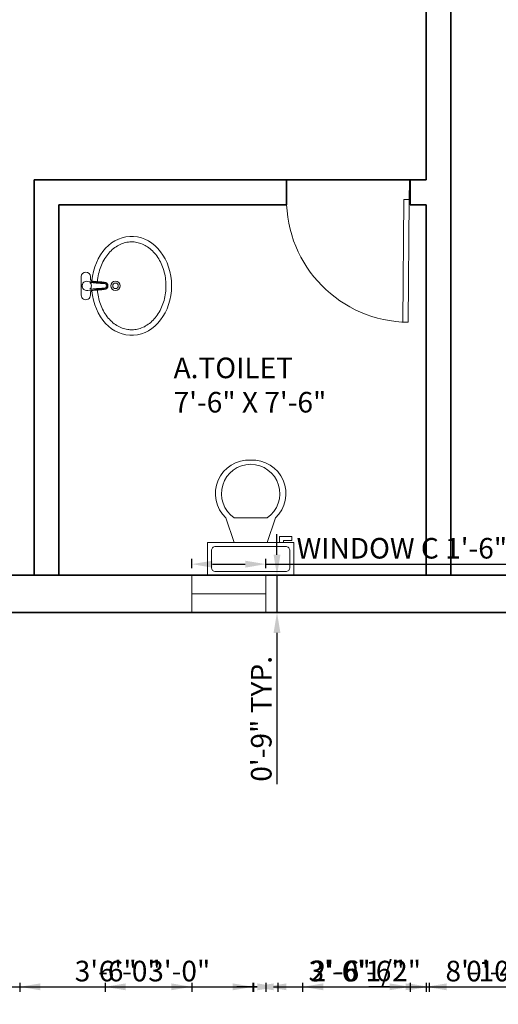
# Model space of a CAD drawing. Units: inches. Extents: x -100 to 766, y -562 to 63.
# Tile 2 of 11: x 152 to 268, y -562 to -323. Entities that reach past the tile are written whole.
import ezdxf

# ---------------------------------------------------------------- set-up
doc = ezdxf.new("R2010")
doc.units = ezdxf.units.IN
for name, color, linetype, lineweight in [('A-ANNO-DIMS', 2, 'Continuous', 18), ('A-AREA-IDEN', 7, 'Continuous', 18), ('A-DOOR', 3, 'Continuous', 18), ('A-FLOR-FIXT', 8, 'Continuous', 18), ('A-GLAZ', 4, 'Continuous', 18), ('A-WALL', 7, 'Continuous', 35)]:
    doc.layers.add(name, color=color, linetype=linetype, lineweight=lineweight)
doc.styles.get("Standard").update_dxf_attribs({"font": 'arial.ttf'})
doc.dimstyles.new('ISO-25', dxfattribs={"dimtxt": 5, "dimasz": 5, "dimexe": 1.25, "dimexo": 0.625, "dimtad": 1, "dimlunit": 3, "dimtxsty": 'Standard', "dimcen": 2.5, "dimadec": 0, "dimazin": 0, "dimtfac": 1, "dimtmove": 0, "dimatfit": 3, "dimfxl": 1, "dimfxlon": 1, "dimarcsym": 0})

# ---------------------------------------------------------------- blocks, each defined once
blk = doc.blocks.new('*U2')
for p, q in [((0, 0), (0, -6)), ((40, 0), (40, -6))]:
    blk.add_line(p, q)
blk.add_lwpolyline([(0, 0), (0, 40), (1.75, 40), (1.75, 0)], close=True)
blk.add_arc((0, 0), 40, 0, 90)
blk = doc.blocks.new('*U4')
for p, q in [((9.5, -6), (9.5, -2)), ((-10, -8.5), (-8, -8.5)), ((-10, -9.5), (-10, -8.5)), ((-7, -9.5), (-10, -9.5)), ((-8, -8.5), (-8, -8)), ((-7, -8), (-7, -9.5)), ((-4, -8), (-6, -14)), ((4, -8), (6, -14)), ((4, -14), (-4, -14))]:
    blk.add_line(p, q)
blk.add_lwpolyline([(10.5, -8), (10.5, 0), (-10.5, 0), (-10.5, -8)], close=True)
for points in [[(-9.5, -2), (-9.5, -6)], [(8.5, -1), (-8.5, -1)], [(-8.5, -7), (8.5, -7)]]:
    blk.add_lwpolyline(points)
for centre, radius, start, end in [((-8.625, -1.875), 0.8839, 81.8699, 188.1301), ((8.625, -1.875), 0.8839, 351.8699, 98.1301), ((-8.625, -6.125), 0.8839, 171.869898, 278.1301), ((8.625, -6.125), 0.8839, 261.8699, 8.1301), ((-0.4772, -19.9188), 8.0953, 133.01722, 273.38), ((0.0374, -19.8731), 7.127, 124.50543, 269.7), ((-0.0373, -19.8731), 7.127, 270.3, 55.4946), ((0.4773, -19.9188), 8.0953, 266.62, 46.9828)]:
    blk.add_arc(centre, radius, start, end)
blk = doc.blocks.new('A$C359865C9')
for p, q in [((0.26, 0.5858), (0.38, 0.5858)), ((0.26, 0.5258), (0.272, 0.5258)), ((0.368, 0.5258), (0.3809, 0.5258))]:
    blk.add_line(p, q)
for radius in [0.03, 0.018]:
    blk.add_circle((0.3201, 0.3632), radius)
for centre, radius, start, end in [((0.26, 0.5558), 0.03, 90.00613, 270.00613), ((0.32, 0.5495), 0.03, 348.15369, 191.84631), ((0.38, 0.5558), 0.03, 270.00613, 89.98161), ((0.272, 0.5078), 0.018, 0.00613, 90.00613), ((0.32, 0.5495), 0.03, 222.45226, 317.54774), ((0.368, 0.5078), 0.018, 90.00613, 180.00613), ((0.3201, 0.4358), 0.024, 180.00613, 0.00613), ((0.3201, 0.4358), 0.0204, 180.00613, 0.00613), ((0.3201, 0.4358), 0.0144, 180.00613, 0.00613)]:
    blk.add_arc(centre, radius, start, end)
at = {"extrusion": (0, 0, -1)}
blk.add_ellipse((0.3199, 0.5826), major_axis=(-0.00812, 0), ratio=0.392595, dxfattribs=at)
at = {"ltscale": 100, "extrusion": (0, 0, -1)}
blk.add_ellipse((0.3201, 0.258), major_axis=(0.3216, 0), ratio=0.80597, start_param=-1.471508, end_param=4.612925, dxfattribs=at)
for points, knots in [([(0.2907, 0.5434), (0.2946, 0.498), (0.2952, 0.4908), (0.2965, 0.4761), (0.2971, 0.4686), (0.2983, 0.4536), (0.2989, 0.4461), (0.2995, 0.4378), (0.2996, 0.4369), (0.2996, 0.4361)], [2.511178, 2.511178, 2.511178, 2.511178, 20.495008, 20.495008, 39.297594, 39.297594, 58.10018, 58.10018, 60.208758, 60.208758, 60.208758, 60.208758]), ([(0.2979, 0.5293), (0.298, 0.528), (0.2981, 0.5267), (0.2988, 0.5184), (0.2993, 0.5127), (0.3005, 0.4986), (0.301, 0.4933), (0.3014, 0.4884), (0.3015, 0.4875), (0.3017, 0.4857), (0.3017, 0.485), (0.3019, 0.4827), (0.3021, 0.4812), (0.3026, 0.4756), (0.3029, 0.4716), (0.3037, 0.4621), (0.3041, 0.4568), (0.3049, 0.4464), (0.3053, 0.4415), (0.3056, 0.4365)], [4.643985, 4.643985, 4.643985, 4.643985, 5.282102, 5.282102, 8.976667, 8.976667, 16.365798, 16.365798, 18.536065, 18.536065, 20.434607, 20.434607, 24.231692, 24.231692, 34.371999, 34.371999, 47.807513, 47.807513, 60.208758, 60.208758, 60.208758, 60.208758]), ([(0.3422, 0.5293), (0.3421, 0.528), (0.342, 0.5267), (0.3412, 0.5184), (0.3408, 0.5127), (0.3395, 0.4986), (0.3391, 0.4933), (0.3387, 0.4884), (0.3386, 0.4875), (0.3384, 0.4857), (0.3383, 0.485), (0.3381, 0.4827), (0.338, 0.4812), (0.3375, 0.4756), (0.3372, 0.4716), (0.3364, 0.4621), (0.336, 0.4568), (0.3352, 0.4464), (0.3348, 0.4415), (0.3345, 0.4365)], [4.643985, 4.643985, 4.643985, 4.643985, 5.282102, 5.282102, 8.976667, 8.976667, 16.365798, 16.365798, 18.536065, 18.536065, 20.434607, 20.434607, 24.231692, 24.231692, 34.371999, 34.371999, 47.807513, 47.807513, 60.208758, 60.208758, 60.208758, 60.208758]), ([(0.3494, 0.5434), (0.3455, 0.498), (0.3449, 0.4908), (0.3436, 0.4761), (0.343, 0.4686), (0.3418, 0.4536), (0.3412, 0.4461), (0.3406, 0.4378), (0.3405, 0.4369), (0.3404, 0.4361)], [2.511178, 2.511178, 2.511178, 2.511178, 20.495008, 20.495008, 39.297594, 39.297594, 58.10018, 58.10018, 60.208758, 60.208758, 60.208758, 60.208758]), ([(0.3475, 0.4801), (0.3477, 0.4801), (0.3479, 0.4801), (0.3648, 0.4788), (0.3813, 0.4763), (0.4136, 0.4692), (0.4293, 0.4645), (0.4593, 0.4531), (0.4737, 0.4464), (0.5006, 0.4312), (0.5131, 0.4227), (0.5361, 0.4042), (0.5465, 0.3942), (0.5649, 0.3732), (0.5729, 0.3622), (0.5864, 0.3393), (0.5918, 0.3275), (0.6, 0.3036), (0.6029, 0.2914), (0.6059, 0.2669), (0.6061, 0.2545), (0.6039, 0.2301), (0.6015, 0.218), (0.5941, 0.1942), (0.5892, 0.1825), (0.5768, 0.1597), (0.5693, 0.1486), (0.552, 0.1275), (0.5422, 0.1174), (0.5203, 0.0986), (0.5083, 0.0899), (0.4825, 0.0741), (0.4686, 0.0671), (0.4396, 0.0549), (0.4243, 0.0498), (0.3929, 0.0418), (0.3767, 0.0388), (0.3439, 0.0352), (0.3273, 0.0344), (0.2942, 0.0353), (0.2776, 0.0369), (0.2452, 0.0422), (0.2293, 0.046), (0.1987, 0.0556), (0.1839, 0.0615), (0.156, 0.0751), (0.1428, 0.0828), (0.1184, 0.0997), (0.1071, 0.109), (0.0869, 0.1288), (0.078, 0.1393), (0.0625, 0.1611), (0.0559, 0.1725), (0.0454, 0.1957), (0.0415, 0.2076), (0.036, 0.2317), (0.0346, 0.2438), (0.0345, 0.2566), (0.0345, 0.2573), (0.0345, 0.258), (0.0345, 0.2664), (0.0351, 0.2749), (0.0382, 0.2956), (0.0413, 0.3078), (0.0502, 0.3317), (0.0559, 0.3434), (0.0699, 0.3661), (0.0782, 0.377), (0.0972, 0.3978), (0.1079, 0.4076), (0.1313, 0.4257), (0.1441, 0.434), (0.1714, 0.4488), (0.186, 0.4553), (0.2163, 0.4662), (0.2321, 0.4706), (0.2628, 0.4769), (0.2776, 0.479), (0.2925, 0.4801)], [1.664851, 1.664851, 1.664851, 1.664851, 1.666804, 1.666804, 1.838807, 1.838807, 2.01081, 2.01081, 2.182814, 2.182814, 2.354817, 2.354817, 2.52682, 2.52682, 2.698824, 2.698824, 2.870827, 2.870827, 3.04283, 3.04283, 3.214834, 3.214834, 3.384783, 3.384783, 3.554732, 3.554732, 3.724681, 3.724681, 3.89463, 3.89463, 4.064578, 4.064578, 4.234527, 4.234527, 4.404476, 4.404476, 4.574425, 4.574425, 4.744374, 4.744374, 4.914323, 4.914323, 5.084272, 5.084272, 5.254221, 5.254221, 5.42417, 5.42417, 5.594119, 5.594119, 5.764068, 5.764068, 5.934016, 5.934016, 6.103965, 6.103965, 6.273914, 6.273914, 6.283185, 6.283185, 6.283185, 6.401959, 6.401959, 6.573962, 6.573962, 6.745965, 6.745965, 6.917969, 6.917969, 7.089972, 7.089972, 7.261975, 7.261975, 7.433979, 7.433979, 7.605982, 7.605982, 7.759676, 7.759676, 7.759676, 7.759676]), ([(0.29, 0.5078), (0.2913, 0.4937), (0.2935, 0.4697), (0.2953, 0.4457), (0.2961, 0.4358)], [0, 0, 0, 0, 35.358253, 60.208758, 60.208758, 60.208758, 60.208758]), ([(0.35, 0.5078), (0.3487, 0.4937), (0.3466, 0.4697), (0.3448, 0.4457), (0.344, 0.4358)], [0, 0, 0, 0, 35.358253, 60.208758, 60.208758, 60.208758, 60.208758])]:
    blk.add_open_spline(points, degree=3, knots=knots)
blk = doc.blocks.new('WIN-18IN')
blk.add_line((4.5, 18), (4.5, 0))
blk.add_lwpolyline([(0, 18), (9, 18), (9, 0), (0, 0)], close=True)
blk = doc.blocks.new('*D22')
at = {"layer": 'A-ANNO-DIMS', "color": 0, "lineweight": -2, "transparency": 16777216}
for p, q in [((193.47, -456.51), (193.47, -454.26)), ((211.47, -456.51), (211.47, -454.26)), ((198.47, -455.51), (206.47, -455.51)), ((211.47, -455.51), (287.98, -455.51))]:
    blk.add_line(p, q, dxfattribs=at)
at = {"layer": 'A-ANNO-DIMS', "color": 0, "transparency": 16777216}
for points in [[(198.47, -454.68), (198.47, -456.35), (193.47, -455.51)], [(206.47, -454.68), (206.47, -456.35), (211.47, -455.51)]]:
    blk.add_solid(points, dxfattribs=at)
at = {"layer": 'Defpoints', "color": 0, "transparency": 16777216}
for p in [(211.47, -455.51), (193.47, -458.21), (211.47, -458.21)]:
    blk.add_point(p, dxfattribs=at)
at = {"layer": 'A-ANNO-DIMS', "color": 0, "transparency": 16777216, "insert": (252.23, -452.3), "char_height": 5, "attachment_point": 5}
blk.add_mtext('WINDOW C 1\'-6" TYP.', dxfattribs=at)
blk = doc.blocks.new('*D23')
at = {"layer": 'A-ANNO-DIMS', "color": 0, "lineweight": -2, "transparency": 16777216}
for p, q in [((214.17, -453.21), (214.17, -448.21)), ((213.17, -458.21), (215.42, -458.21)), ((214.17, -458.21), (214.17, -467.21)), ((213.17, -467.21), (215.42, -467.21)), ((214.17, -472.21), (214.17, -508.94))]:
    blk.add_line(p, q, dxfattribs=at)
at = {"layer": 'A-ANNO-DIMS', "color": 0, "transparency": 16777216}
for points in [[(213.34, -453.21), (215.01, -453.21), (214.17, -458.21)], [(213.34, -472.21), (215.01, -472.21), (214.17, -467.21)]]:
    blk.add_solid(points, dxfattribs=at)
at = {"layer": 'Defpoints', "color": 0, "transparency": 16777216}
for p in [(211.47, -458.21), (211.47, -467.21), (214.17, -467.21)]:
    blk.add_point(p, dxfattribs=at)
at = {"layer": 'A-ANNO-DIMS', "color": 0, "transparency": 16777216, "insert": (211, -493.08), "char_height": 5, "attachment_point": 5, "rotation": 90}
blk.add_mtext('0\'-9" TYP.', dxfattribs=at)
blk = doc.blocks.new('*D40')
at = {"layer": 'A-ANNO-DIMS', "color": 0, "lineweight": -2, "transparency": 16777216}
for p, q in [((142.39, -557.16), (142.39, -559.41)), ((147.39, -558.16), (209.39, -558.16)), ((214.39, -557.16), (214.39, -559.41))]:
    blk.add_line(p, q, dxfattribs=at)
at = {"layer": 'A-ANNO-DIMS', "color": 0, "transparency": 16777216}
for points in [[(147.39, -557.32), (147.39, -558.99), (142.39, -558.16)], [(209.39, -557.32), (209.39, -558.99), (214.39, -558.16)]]:
    blk.add_solid(points, dxfattribs=at)
at = {"layer": 'Defpoints', "color": 0, "transparency": 16777216}
for p in [(142.39, -56.21), (214.39, -56.21), (214.39, -558.16)]:
    blk.add_point(p, dxfattribs=at)
at = {"layer": 'A-ANNO-DIMS', "color": 0, "transparency": 16777216, "insert": (178.39, -554.98), "char_height": 5, "attachment_point": 5}
blk.add_mtext('6\'-0"', dxfattribs=at)
blk = doc.blocks.new('*D46')
at = {"layer": 'A-ANNO-DIMS', "color": 0, "lineweight": -2, "transparency": 16777216}
for p, q in [((209.39, -558.16), (204.39, -558.16)), ((214.39, -557.16), (214.39, -559.41)), ((214.39, -558.16), (220.39, -558.16)), ((220.39, -557.16), (220.39, -559.41)), ((225.39, -558.16), (244.93, -558.16))]:
    blk.add_line(p, q, dxfattribs=at)
at = {"layer": 'A-ANNO-DIMS', "color": 0, "transparency": 16777216}
for points in [[(209.39, -557.32), (209.39, -558.99), (214.39, -558.16)], [(225.39, -557.32), (225.39, -558.99), (220.39, -558.16)]]:
    blk.add_solid(points, dxfattribs=at)
at = {"layer": 'Defpoints', "color": 0, "transparency": 16777216}
for p in [(214.39, -182.21), (220.39, -182.21), (220.39, -558.16)]:
    blk.add_point(p, dxfattribs=at)
at = {"layer": 'A-ANNO-DIMS', "color": 0, "transparency": 16777216, "insert": (237.66, -554.98), "char_height": 5, "attachment_point": 5}
blk.add_mtext('0\'-6"', dxfattribs=at)
blk = doc.blocks.new('*D47')
at = {"layer": 'A-ANNO-DIMS', "color": 0, "lineweight": -2, "transparency": 16777216}
for p, q in [((172.42, -557.16), (172.42, -559.41)), ((177.42, -558.16), (203.43, -558.16)), ((208.43, -557.16), (208.43, -559.41))]:
    blk.add_line(p, q, dxfattribs=at)
at = {"layer": 'A-ANNO-DIMS', "color": 0, "transparency": 16777216}
for points in [[(177.42, -557.32), (177.42, -558.99), (172.42, -558.16)], [(203.43, -557.32), (203.43, -558.99), (208.43, -558.16)]]:
    blk.add_solid(points, dxfattribs=at)
at = {"layer": 'Defpoints', "color": 0, "transparency": 16777216}
for p in [(172.42, -182.21), (208.43, -182.21), (208.43, -558.16)]:
    blk.add_point(p, dxfattribs=at)
at = {"layer": 'A-ANNO-DIMS', "color": 0, "transparency": 16777216, "insert": (190.43, -554.98), "char_height": 5, "attachment_point": 5}
blk.add_mtext('3\'-0"', dxfattribs=at)
blk = doc.blocks.new('*D49')
at = {"layer": 'A-ANNO-DIMS', "color": 0, "lineweight": -2, "transparency": 16777216}
for p, q in [((-88.51, -356.21), (-90.76, -356.21)), ((-89.51, -361.21), (-89.51, -417.21)), ((-88.51, -422.21), (-90.76, -422.21))]:
    blk.add_line(p, q, dxfattribs=at)
at = {"layer": 'A-ANNO-DIMS', "color": 0, "transparency": 16777216}
for points in [[(-90.35, -361.21), (-88.68, -361.21), (-89.51, -356.21)], [(-90.35, -417.21), (-88.68, -417.21), (-89.51, -422.21)]]:
    blk.add_solid(points, dxfattribs=at)
at = {"layer": 'Defpoints', "color": 0, "transparency": 16777216}
for p in [(562.39, -356.21), (-89.51, -422.21), (562.39, -422.21)]:
    blk.add_point(p, dxfattribs=at)
at = {"layer": 'A-ANNO-DIMS', "color": 0, "transparency": 16777216, "insert": (-92.69, -389.21), "char_height": 5, "attachment_point": 5, "rotation": 90}
blk.add_mtext('5\'-6"', dxfattribs=at)
blk = doc.blocks.new('*D51')
at = {"layer": 'A-ANNO-DIMS', "color": 0, "lineweight": -2, "transparency": 16777216}
for p, q in [((-88.51, -308.21), (-90.76, -308.21)), ((-89.51, -313.21), (-89.51, -339.21)), ((-88.51, -344.21), (-90.76, -344.21))]:
    blk.add_line(p, q, dxfattribs=at)
at = {"layer": 'A-ANNO-DIMS', "color": 0, "transparency": 16777216}
for points in [[(-90.35, -313.21), (-88.68, -313.21), (-89.51, -308.21)], [(-90.35, -339.21), (-88.68, -339.21), (-89.51, -344.21)]]:
    blk.add_solid(points, dxfattribs=at)
at = {"layer": 'Defpoints', "color": 0, "transparency": 16777216}
for p in [(598.6, -308.21), (-89.51, -344.21), (598.6, -344.21)]:
    blk.add_point(p, dxfattribs=at)
at = {"layer": 'A-ANNO-DIMS', "color": 0, "transparency": 16777216, "insert": (-92.69, -326.21), "char_height": 5, "attachment_point": 5, "rotation": 90}
blk.add_mtext('3\'-0"', dxfattribs=at)
blk = doc.blocks.new('*D56')
at = {"layer": 'A-ANNO-DIMS', "color": 0, "lineweight": -2, "transparency": 16777216}
for p, q in [((220.39, -557.16), (220.39, -559.41)), ((225.39, -558.16), (246.11, -558.16)), ((251.11, -557.16), (251.11, -559.41))]:
    blk.add_line(p, q, dxfattribs=at)
at = {"layer": 'A-ANNO-DIMS', "color": 0, "transparency": 16777216}
for points in [[(225.39, -557.32), (225.39, -558.99), (220.39, -558.16)], [(246.11, -557.32), (246.11, -558.99), (251.11, -558.16)]]:
    blk.add_solid(points, dxfattribs=at)
at = {"layer": 'Defpoints', "color": 0, "transparency": 16777216}
for p in [(220.39, -159.2), (251.11, -159.2), (251.11, -558.16)]:
    blk.add_point(p, dxfattribs=at)
at = {"layer": 'A-ANNO-DIMS', "color": 0, "transparency": 16777216, "insert": (235.75, -554.95), "char_height": 5, "attachment_point": 5}
blk.add_mtext('2\'-6 1/2"', dxfattribs=at)
blk = doc.blocks.new('*D66')
at = {"layer": 'A-ANNO-DIMS', "color": 0, "lineweight": -2, "transparency": 16777216}
for p, q in [((151.67, -557.16), (151.67, -559.41)), ((156.67, -558.16), (188.47, -558.16)), ((193.47, -557.16), (193.47, -559.41))]:
    blk.add_line(p, q, dxfattribs=at)
at = {"layer": 'A-ANNO-DIMS', "color": 0, "transparency": 16777216}
for points in [[(156.67, -557.32), (156.67, -558.99), (151.67, -558.16)], [(188.47, -557.32), (188.47, -558.99), (193.47, -558.16)]]:
    blk.add_solid(points, dxfattribs=at)
at = {"layer": 'Defpoints', "color": 0, "transparency": 16777216}
for p in [(151.67, -467.19), (193.47, -467.21), (193.47, -558.16)]:
    blk.add_point(p, dxfattribs=at)
at = {"layer": 'A-ANNO-DIMS', "color": 0, "transparency": 16777216, "insert": (172.57, -554.98), "char_height": 5, "attachment_point": 5}
blk.add_mtext('3\'-6"', dxfattribs=at)
blk = doc.blocks.new('*D67')
at = {"layer": 'A-ANNO-DIMS', "color": 0, "lineweight": -2, "transparency": 16777216}
for p, q in [((211.47, -557.16), (211.47, -559.41)), ((216.47, -558.16), (312.6, -558.16)), ((317.6, -557.16), (317.6, -559.41))]:
    blk.add_line(p, q, dxfattribs=at)
at = {"layer": 'A-ANNO-DIMS', "color": 0, "transparency": 16777216}
for points in [[(216.47, -557.32), (216.47, -558.99), (211.47, -558.16)], [(312.6, -557.32), (312.6, -558.99), (317.6, -558.16)]]:
    blk.add_solid(points, dxfattribs=at)
at = {"layer": 'Defpoints', "color": 0, "transparency": 16777216}
for p in [(211.47, -467.21), (317.6, -467.21), (317.6, -558.16)]:
    blk.add_point(p, dxfattribs=at)
at = {"layer": 'A-ANNO-DIMS', "color": 0, "transparency": 16777216, "insert": (264.53, -554.98), "char_height": 5, "attachment_point": 5}
blk.add_mtext('8\'-10"', dxfattribs=at)
blk = doc.blocks.new('*D70')
at = {"layer": 'A-ANNO-DIMS', "color": 0, "lineweight": -2, "transparency": 16777216}
for p, q in [((-88.51, -376.85), (-90.76, -376.85)), ((-89.51, -381.85), (-89.51, -419.34)), ((-88.51, -424.34), (-90.76, -424.34))]:
    blk.add_line(p, q, dxfattribs=at)
at = {"layer": 'A-ANNO-DIMS', "color": 0, "transparency": 16777216}
for points in [[(-90.35, -381.85), (-88.68, -381.85), (-89.51, -376.85)], [(-90.35, -419.34), (-88.68, -419.34), (-89.51, -424.34)]]:
    blk.add_solid(points, dxfattribs=at)
at = {"layer": 'Defpoints', "color": 0, "transparency": 16777216}
for p in [(679.5, -376.85), (-89.51, -424.34), (679.5, -424.34)]:
    blk.add_point(p, dxfattribs=at)
at = {"layer": 'A-ANNO-DIMS', "color": 0, "transparency": 16777216, "insert": (-92.73, -400.59), "char_height": 5, "attachment_point": 5, "rotation": 90}
blk.add_mtext('3\'-11 1/2"', dxfattribs=at)
blk = doc.blocks.new('*D73')
at = {"layer": 'A-ANNO-DIMS', "color": 0, "lineweight": -2, "transparency": 16777216}
for p, q in [((-88.51, -345.04), (-90.76, -345.04)), ((-89.51, -350.04), (-89.51, -401.82)), ((-88.51, -406.82), (-90.76, -406.82))]:
    blk.add_line(p, q, dxfattribs=at)
at = {"layer": 'A-ANNO-DIMS', "color": 0, "transparency": 16777216}
for points in [[(-90.35, -350.04), (-88.68, -350.04), (-89.51, -345.04)], [(-90.35, -401.82), (-88.68, -401.82), (-89.51, -406.82)]]:
    blk.add_solid(points, dxfattribs=at)
at = {"layer": 'Defpoints', "color": 0, "transparency": 16777216}
for p in [(475.3, -345.04), (-89.51, -406.82), (475.3, -406.82)]:
    blk.add_point(p, dxfattribs=at)
at = {"layer": 'A-ANNO-DIMS', "color": 0, "transparency": 16777216, "insert": (-92.69, -375.93), "char_height": 5, "attachment_point": 5, "rotation": 90}
blk.add_mtext('5\'-2"', dxfattribs=at)
blk = doc.blocks.new('*D78')
at = {"layer": 'A-ANNO-DIMS', "color": 0, "lineweight": -2, "transparency": 16777216}
for p, q in [((208.34, -557.16), (208.34, -559.41)), ((213.34, -558.16), (245.39, -558.16)), ((250.39, -557.16), (250.39, -559.41))]:
    blk.add_line(p, q, dxfattribs=at)
at = {"layer": 'A-ANNO-DIMS', "color": 0, "transparency": 16777216}
for points in [[(213.34, -557.32), (213.34, -558.99), (208.34, -558.16)], [(245.39, -557.32), (245.39, -558.99), (250.39, -558.16)]]:
    blk.add_solid(points, dxfattribs=at)
at = {"layer": 'Defpoints', "color": 0, "transparency": 16777216}
for p in [(208.34, -278.21), (250.39, -278.21), (250.39, -558.16)]:
    blk.add_point(p, dxfattribs=at)
at = {"layer": 'A-ANNO-DIMS', "color": 0, "transparency": 16777216, "insert": (229.37, -554.98), "char_height": 5, "attachment_point": 5}
blk.add_mtext('3\'-6"', dxfattribs=at)
blk = doc.blocks.new('*D79')
at = {"layer": 'A-ANNO-DIMS', "color": 0, "lineweight": -2, "transparency": 16777216}
for p, q in [((216.52, 51.68), (216.52, 53.93)), ((221.52, 52.68), (241.52, 52.68)), ((246.52, 51.68), (246.52, 53.93))]:
    blk.add_line(p, q, dxfattribs=at)
at = {"layer": 'A-ANNO-DIMS', "color": 0, "transparency": 16777216}
for points in [[(221.52, 53.51), (221.52, 51.84), (216.52, 52.68)], [(241.52, 53.51), (241.52, 51.84), (246.52, 52.68)]]:
    blk.add_solid(points, dxfattribs=at)
at = {"layer": 'Defpoints', "color": 0, "transparency": 16777216}
for p in [(246.52, 52.68), (216.52, -362.21), (246.52, -362.21)]:
    blk.add_point(p, dxfattribs=at)
at = {"layer": 'A-ANNO-DIMS', "color": 0, "transparency": 16777216, "insert": (231.52, 55.86), "char_height": 5, "attachment_point": 5}
blk.add_mtext('2\'-6"', dxfattribs=at)
blk = doc.blocks.new('*D80')
at = {"layer": 'A-ANNO-DIMS', "color": 0, "lineweight": -2, "transparency": 16777216}
for p, q in [((241.52, -558.16), (236.52, -558.16)), ((246.52, -557.16), (246.52, -559.41)), ((246.52, -558.16), (250.39, -558.16)), ((250.39, -557.16), (250.39, -559.41)), ((255.39, -558.16), (274.93, -558.16))]:
    blk.add_line(p, q, dxfattribs=at)
at = {"layer": 'A-ANNO-DIMS', "color": 0, "transparency": 16777216}
for points in [[(241.52, -557.32), (241.52, -558.99), (246.52, -558.16)], [(255.39, -557.32), (255.39, -558.99), (250.39, -558.16)]]:
    blk.add_solid(points, dxfattribs=at)
at = {"layer": 'Defpoints', "color": 0, "transparency": 16777216}
for p in [(246.52, -368.21), (250.39, -368.21), (250.39, -558.16)]:
    blk.add_point(p, dxfattribs=at)
at = {"layer": 'A-ANNO-DIMS', "color": 0, "transparency": 16777216, "insert": (267.66, -554.98), "char_height": 5, "attachment_point": 5}
blk.add_mtext('0\'-4"', dxfattribs=at)
blk = doc.blocks.new('*D83')
at = {"layer": 'A-ANNO-DIMS', "color": 0, "lineweight": -2, "transparency": 16777216}
for p, q in [((-88.51, -422.21), (-90.76, -422.21)), ((-89.51, -427.21), (-89.51, -453.21)), ((-88.51, -458.21), (-90.76, -458.21))]:
    blk.add_line(p, q, dxfattribs=at)
at = {"layer": 'A-ANNO-DIMS', "color": 0, "transparency": 16777216}
for points in [[(-90.35, -427.21), (-88.68, -427.21), (-89.51, -422.21)], [(-90.35, -453.21), (-88.68, -453.21), (-89.51, -458.21)]]:
    blk.add_solid(points, dxfattribs=at)
at = {"layer": 'Defpoints', "color": 0, "transparency": 16777216}
for p in [(562.39, -422.21), (-89.51, -458.21), (562.39, -458.21)]:
    blk.add_point(p, dxfattribs=at)
at = {"layer": 'A-ANNO-DIMS', "color": 0, "transparency": 16777216, "insert": (-92.69, -440.21), "char_height": 5, "attachment_point": 5, "rotation": 90}
blk.add_mtext('3\'-0"', dxfattribs=at)

msp = doc.modelspace()

# ---------------------------------------------------------------- linework, layer by layer
at = {"layer": 'A-WALL'}
for p, q in [((256.388, -458.214), (256.388, -272.214)), ((250.388, -362.214), (250.388, -278.214)), ((155.218, -362.214), (250.388, -362.214)), ((155.218, -368.214), (155.218, -362.214)), ((216.522, -362.214), (216.522, -368.214)), ((246.522, -362.214), (246.522, -368.214)), ((155.218, -458.214), (155.218, -368.214)), ((161.218, -458.214), (161.218, -368.214)), ((161.218, -368.214), (216.522, -368.214)), ((246.522, -368.214), (250.388, -368.214)), ((250.388, -458.214), (250.388, -368.214)), ((250.388, -458.214), (10.388, -458.214)), ((532.388, -458.214), (250.388, -458.214))]:
    msp.add_line(p, q, dxfattribs=at)
msp.add_lwpolyline([(1.388, 12.786), (721.388, 12.786), (721.388, -467.214), (1.388, -467.214)], close=True, dxfattribs=at)

# ---------------------------------------------------------------- block references
at = {"layer": 'A-DOOR', "xscale": 0.7457426098631386, "yscale": 0.7457426098631386, "zscale": 0.7457426098631386, "rotation": 179.5326886568227}
msp.add_blockref('*U2', (246.314, -366.932), dxfattribs=at)
at = {"layer": 'A-FLOR-FIXT', "xscale": 37.38131337077302, "yscale": 37.38131337077302, "zscale": 37.38131337077302, "rotation": 90}
msp.add_blockref('A$C359865C9', (188.509, -399.891), dxfattribs=at)
at = {"layer": 'A-FLOR-FIXT', "rotation": 180}
msp.add_blockref('*U4', (207.774, -458.264), dxfattribs=at)
at = {"layer": 'A-GLAZ', "rotation": 270.0000000000005}
msp.add_blockref('WIN-18IN', (193.473, -458.215), dxfattribs=at)

# ---------------------------------------------------------------- texts
at = {"layer": 'A-AREA-IDEN', "insert": (189.059, -405.353), "char_height": 5, "attachment_point": 1}
msp.add_mtext_dynamic_manual_height_columns('A.TOILET\\P7\'-6" X 7\'-6"', width=42.34603, gutter_width=12.5, heights=[0], dxfattribs=at)

# ---------------------------------------------------------------- dimensions: what is measured, and where the dimension line sits
at = {"layer": 'A-ANNO-DIMS'}
for base, p1, p2, picture, middle in [((246.522, 52.678), (216.522, -362.214), (246.522, -362.214), '*D79', (231.522, 55.855)), ((214.388, -558.156), (142.388, -56.214), (214.388, -56.214), '*D40', (178.388, -554.979)), ((251.108, -558.156), (220.388, -159.197), (251.108, -159.197), '*D56', (235.748, -554.946)), ((208.434, -558.156), (172.417, -182.214), (208.434, -182.214), '*D47', (190.425, -554.977)), ((220.388, -558.156), (214.388, -182.214), (220.388, -182.214), '*D46', (237.658, -554.979)), ((250.388, -558.156), (208.344, -278.214), (250.388, -278.214), '*D78', (229.366, -554.977)), ((250.388, -558.156), (246.522, -368.214), (250.388, -368.214), '*D80', (267.658, -554.979)), ((193.473, -558.156), (151.67, -467.193), (193.473, -467.214), '*D66', (172.572, -554.977)), ((317.595, -558.156), (211.473, -467.214), (317.595, -467.214), '*D67', (264.534, -554.979))]:
    dim = msp.add_linear_dim(base=base, p1=p1, p2=p2, dimstyle='ISO-25', override={"dimdec": 1, "dimlfac": 1, "dimrnd": 0, "dimzin": 1, "dimdsep": 46, "dimlunit": 4, "dimfrac": 2}, dxfattribs=at)
    dim.commit()
    dim.dimension.update_dxf_attribs({"geometry": picture, "text_midpoint": middle})
for base, p1, p2, picture, middle in [((-89.513, -344.214), (598.603, -308.214), (598.603, -344.214), '*D51', (-92.693, -326.214)), ((-89.513, -406.822), (475.3, -345.045), (475.3, -406.822), '*D73', (-92.691, -375.933)), ((-89.513, -422.214), (562.394, -356.214), (562.394, -422.214), '*D49', (-92.691, -389.214)), ((-89.513, -424.336), (679.495, -376.848), (679.495, -424.336), '*D70', (-92.725, -400.592)), ((-89.513, -458.214), (562.394, -422.214), (562.394, -458.214), '*D83', (-92.693, -440.214))]:
    dim = msp.add_linear_dim(base=base, p1=p1, p2=p2, angle=90, dimstyle='ISO-25', override={"dimdec": 1, "dimlfac": 1, "dimrnd": 0, "dimzin": 1, "dimdsep": 46, "dimlunit": 4, "dimfrac": 2}, dxfattribs=at)
    dim.commit()
    dim.dimension.update_dxf_attribs({"geometry": picture, "text_midpoint": middle})
for base, p1, p2, angle, text, picture, middle in [((211.473, -455.514), (193.473, -458.214), (211.473, -458.214), 0, 'WINDOW C <> TYP.', '*D22', (252.226, -452.302)), ((214.173, -467.214), (211.473, -458.214), (211.473, -467.214), 270, '<> TYP.', '*D23', (210.995, -493.078))]:
    dim = msp.add_linear_dim(base=base, p1=p1, p2=p2, angle=angle, text=text, dimstyle='ISO-25', override={"dimdec": 1, "dimlfac": 1, "dimrnd": 0, "dimzin": 1, "dimdsep": 46, "dimlunit": 4, "dimfrac": 2}, dxfattribs=at)
    dim.commit()
    dim.dimension.update_dxf_attribs({"geometry": picture, "text_midpoint": middle})

doc.saveas('drawing.dxf')
